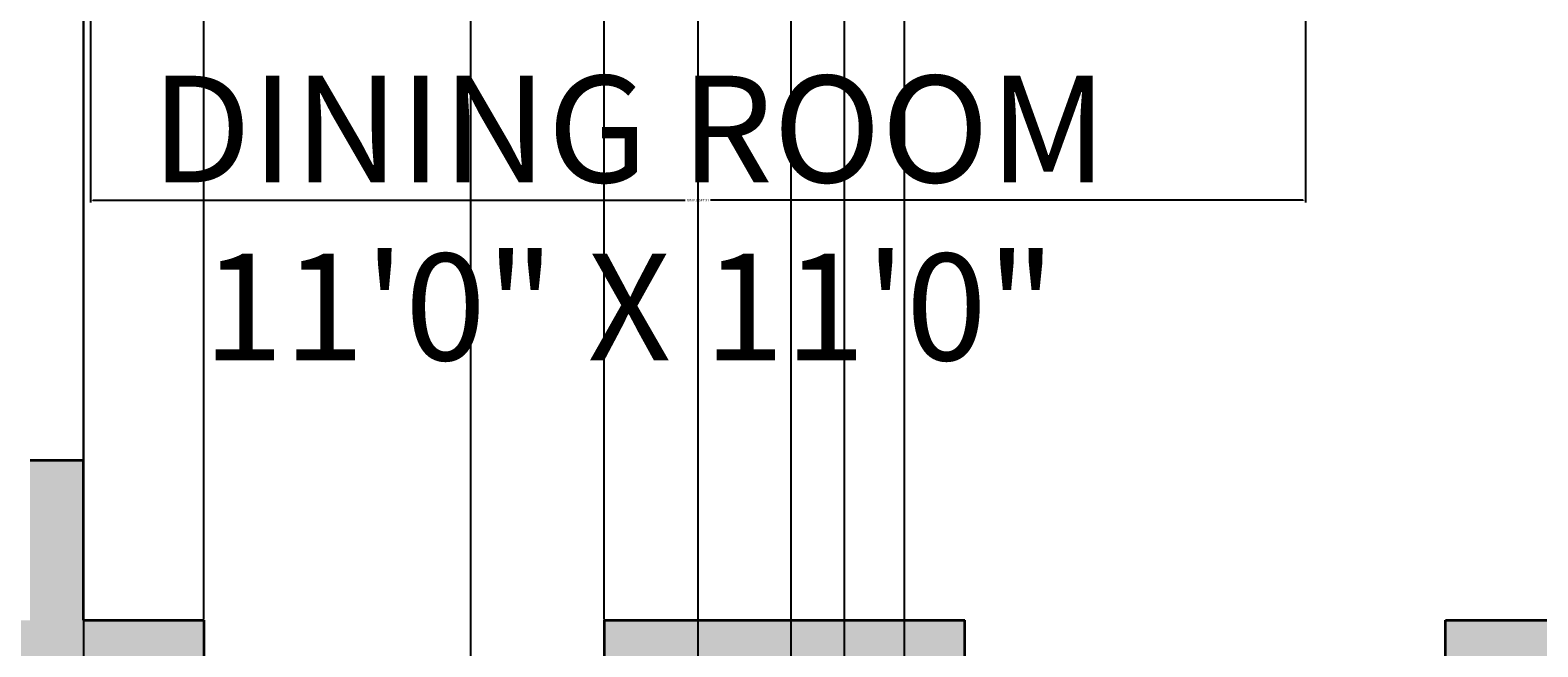
# Model space of a CAD drawing. Units: inches. Extents: x 1567 to 1964, y 1813 to 2447.
# Tile 16 of 28: x 1738 to 1851, y 2125 to 2172. Entities that reach past the tile are written whole.
import ezdxf

# ---------------------------------------------------------------- set-up
doc = ezdxf.new("R2010")
doc.units = ezdxf.units.IN
for name, color, linetype, lineweight in [('A-ANNO-DIMS', 2, 'Continuous', 18), ('A-AREA-IDEN', 7, 'Continuous', 18), ('A-WALL', 7, 'Continuous', 35)]:
    doc.layers.add(name, color=color, linetype=linetype, lineweight=lineweight)
doc.layers.add('A-WALL-PATT', color=251, linetype='Continuous', lineweight=13, true_color=0x636466)
doc.styles.get("Standard").update_dxf_attribs({"font": 'arial.ttf'})
doc.dimstyles.get("Standard").update_dxf_attribs({"dimtxt": 0.18, "dimasz": 0.18, "dimexe": 0.18, "dimexo": 0.0625, "dimgap": 0.09, "dimtad": 0, "dimtih": 1, "dimtoh": 1, "dimdec": 4, "dimzin": 0, "dimdsep": 46, "dimtxsty": 'Standard', "dimcen": 0.09, "dimadec": 0, "dimazin": 0, "dimtfac": 1, "dimtdec": 4, "dimtofl": 0, "dimtmove": 0, "dimatfit": 3, "dimfxl": 1, "dimtolj": 1, "dimtzin": 0, "dimarcsym": 0})

# ---------------------------------------------------------------- blocks, each defined once
blk = doc.blocks.new('*D27')
at = {"layer": 'A-ANNO-DIMS', "color": 0, "lineweight": -2, "transparency": 16777216}
for p, q in [((1742.95, 2172.36), (1742.95, 2158.59)), ((1833.95, 2172.36), (1833.95, 2158.59)), ((1743.13, 2158.77), (1787.5, 2158.77)), ((1833.77, 2158.77), (1789.4, 2158.77))]:
    blk.add_line(p, q, dxfattribs=at)
at = {"layer": 'A-ANNO-DIMS', "color": 0, "transparency": 16777216}
for points in [[(1743.13, 2158.8), (1743.13, 2158.74), (1742.95, 2158.77)], [(1833.77, 2158.8), (1833.77, 2158.74), (1833.95, 2158.77)]]:
    blk.add_solid(points, dxfattribs=at)
at = {"layer": 'Defpoints', "color": 0, "transparency": 16777216}
for p in [(1742.95, 2172.42), (1833.95, 2172.42), (1833.95, 2158.77)]:
    blk.add_point(p, dxfattribs=at)
at = {"layer": 'A-ANNO-DIMS', "color": 0, "transparency": 16777216, "insert": (1788.45, 2158.77), "char_height": 0.18, "attachment_point": 5}
blk.add_mtext('\\A1;DINING SET 91', dxfattribs=at)
blk = doc.blocks.new('*D47')
at = {"layer": 'A-ANNO-DIMS', "color": 0, "lineweight": -2, "transparency": 16777216}
for p, q in [((1742.43, 2331.23), (1742.43, 1813.46)), ((1788.43, 2331.23), (1788.43, 1813.46)), ((1742.61, 1813.64), (1765.21, 1813.64)), ((1788.25, 1813.64), (1765.65, 1813.64))]:
    blk.add_line(p, q, dxfattribs=at)
at = {"layer": 'A-ANNO-DIMS', "color": 0, "transparency": 16777216}
for points in [[(1742.61, 1813.67), (1742.61, 1813.61), (1742.43, 1813.64)], [(1788.25, 1813.67), (1788.25, 1813.61), (1788.43, 1813.64)]]:
    blk.add_solid(points, dxfattribs=at)
at = {"layer": 'Defpoints', "color": 0, "transparency": 16777216}
for p in [(1742.43, 2331.29), (1788.43, 2331.29), (1788.43, 1813.64)]:
    blk.add_point(p, dxfattribs=at)
at = {"layer": 'A-ANNO-DIMS', "color": 0, "transparency": 16777216, "insert": (1765.43, 1813.64), "char_height": 0.18, "attachment_point": 5}
blk.add_mtext('\\A1;46', dxfattribs=at)
blk = doc.blocks.new('*D54')
at = {"layer": 'A-ANNO-DIMS', "color": 0, "lineweight": -2, "transparency": 16777216}
for p, q in [((1711.43, 1964.35), (1711.43, 2447.12)), ((1711.61, 2446.94), (1753.21, 2446.94)), ((1795.25, 2446.94), (1753.65, 2446.94)), ((1795.43, 1964.35), (1795.43, 2447.12))]:
    blk.add_line(p, q, dxfattribs=at)
at = {"layer": 'A-ANNO-DIMS', "color": 0, "transparency": 16777216}
for points in [[(1711.61, 2446.97), (1711.61, 2446.91), (1711.43, 2446.94)], [(1795.25, 2446.97), (1795.25, 2446.91), (1795.43, 2446.94)]]:
    blk.add_solid(points, dxfattribs=at)
at = {"layer": 'Defpoints', "color": 0, "transparency": 16777216}
for p in [(1795.43, 2446.94), (1711.43, 1964.29), (1795.43, 1964.29)]:
    blk.add_point(p, dxfattribs=at)
at = {"layer": 'A-ANNO-DIMS', "color": 0, "transparency": 16777216, "insert": (1753.43, 2446.94), "char_height": 0.18, "attachment_point": 5}
blk.add_mtext('\\A1;84', dxfattribs=at)
blk = doc.blocks.new('*D55')
at = {"layer": 'A-ANNO-DIMS', "color": 0, "lineweight": -2, "transparency": 16777216}
for p, q in [((1795.43, 1964.35), (1795.43, 2447.12)), ((1795.61, 2446.94), (1797.28, 2446.94)), ((1799.25, 2446.94), (1797.58, 2446.94)), ((1799.43, 1967.35), (1799.43, 2447.12))]:
    blk.add_line(p, q, dxfattribs=at)
at = {"layer": 'A-ANNO-DIMS', "color": 0, "transparency": 16777216}
for points in [[(1795.61, 2446.97), (1795.61, 2446.91), (1795.43, 2446.94)], [(1799.25, 2446.97), (1799.25, 2446.91), (1799.43, 2446.94)]]:
    blk.add_solid(points, dxfattribs=at)
at = {"layer": 'Defpoints', "color": 0, "transparency": 16777216}
for p in [(1799.43, 2446.94), (1799.43, 1967.29), (1795.43, 1964.29)]:
    blk.add_point(p, dxfattribs=at)
at = {"layer": 'A-ANNO-DIMS', "color": 0, "transparency": 16777216, "insert": (1797.43, 2446.94), "char_height": 0.18, "attachment_point": 5}
blk.add_mtext('\\A1;4', dxfattribs=at)
blk = doc.blocks.new('*D58')
at = {"layer": 'A-ANNO-DIMS', "color": 0, "lineweight": -2, "transparency": 16777216}
for p, q in [((1742.43, 2127.35), (1742.43, 2447.12)), ((1742.61, 2446.94), (1746.78, 2446.94)), ((1751.25, 2446.94), (1747.08, 2446.94)), ((1751.43, 2127.35), (1751.43, 2447.12))]:
    blk.add_line(p, q, dxfattribs=at)
at = {"layer": 'A-ANNO-DIMS', "color": 0, "transparency": 16777216}
for points in [[(1742.61, 2446.97), (1742.61, 2446.91), (1742.43, 2446.94)], [(1751.25, 2446.97), (1751.25, 2446.91), (1751.43, 2446.94)]]:
    blk.add_solid(points, dxfattribs=at)
at = {"layer": 'Defpoints', "color": 0, "transparency": 16777216}
for p in [(1751.43, 2446.94), (1742.43, 2127.29), (1751.43, 2127.29)]:
    blk.add_point(p, dxfattribs=at)
at = {"layer": 'A-ANNO-DIMS', "color": 0, "transparency": 16777216, "insert": (1746.93, 2446.94), "char_height": 0.18, "attachment_point": 5}
blk.add_mtext('\\A1;9', dxfattribs=at)
blk = doc.blocks.new('*D59')
at = {"layer": 'A-ANNO-DIMS', "color": 0, "lineweight": -2, "transparency": 16777216}
for p, q in [((1751.43, 2127.35), (1751.43, 2447.12)), ((1751.61, 2446.94), (1766.21, 2446.94)), ((1781.25, 2446.94), (1766.65, 2446.94)), ((1781.43, 2127.35), (1781.43, 2447.12))]:
    blk.add_line(p, q, dxfattribs=at)
at = {"layer": 'A-ANNO-DIMS', "color": 0, "transparency": 16777216}
for points in [[(1751.61, 2446.97), (1751.61, 2446.91), (1751.43, 2446.94)], [(1781.25, 2446.97), (1781.25, 2446.91), (1781.43, 2446.94)]]:
    blk.add_solid(points, dxfattribs=at)
at = {"layer": 'Defpoints', "color": 0, "transparency": 16777216}
for p in [(1781.43, 2446.94), (1751.43, 2127.29), (1781.43, 2127.29)]:
    blk.add_point(p, dxfattribs=at)
at = {"layer": 'A-ANNO-DIMS', "color": 0, "transparency": 16777216, "insert": (1766.43, 2446.94), "char_height": 0.18, "attachment_point": 5}
blk.add_mtext('\\A1;30', dxfattribs=at)
blk = doc.blocks.new('*D63')
at = {"layer": 'A-ANNO-DIMS', "color": 0, "lineweight": -2, "transparency": 16777216}
for p, q in [((1735.43, 1988.35), (1735.43, 2447.12)), ((1735.61, 2446.94), (1753.21, 2446.94)), ((1771.25, 2446.94), (1753.65, 2446.94)), ((1771.43, 1988.35), (1771.43, 2447.12))]:
    blk.add_line(p, q, dxfattribs=at)
at = {"layer": 'A-ANNO-DIMS', "color": 0, "transparency": 16777216}
for points in [[(1735.61, 2446.97), (1735.61, 2446.91), (1735.43, 2446.94)], [(1771.25, 2446.97), (1771.25, 2446.91), (1771.43, 2446.94)]]:
    blk.add_solid(points, dxfattribs=at)
at = {"layer": 'Defpoints', "color": 0, "transparency": 16777216}
for p in [(1771.43, 2446.94), (1735.43, 1988.29), (1771.43, 1988.29)]:
    blk.add_point(p, dxfattribs=at)
at = {"layer": 'A-ANNO-DIMS', "color": 0, "transparency": 16777216, "insert": (1753.43, 2446.94), "char_height": 0.18, "attachment_point": 5}
blk.add_mtext('\\A1;36', dxfattribs=at)
blk = doc.blocks.new('*D70')
at = {"layer": 'A-ANNO-DIMS', "color": 0, "lineweight": -2, "transparency": 16777216}
for p, q in [((1799.43, 1967.35), (1799.43, 2447.12)), ((1799.61, 2446.94), (1801.42, 2446.94)), ((1803.75, 2446.94), (1801.94, 2446.94)), ((1803.93, 1967.35), (1803.93, 2447.12))]:
    blk.add_line(p, q, dxfattribs=at)
at = {"layer": 'A-ANNO-DIMS', "color": 0, "transparency": 16777216}
for points in [[(1799.61, 2446.97), (1799.61, 2446.91), (1799.43, 2446.94)], [(1803.75, 2446.97), (1803.75, 2446.91), (1803.93, 2446.94)]]:
    blk.add_solid(points, dxfattribs=at)
at = {"layer": 'Defpoints', "color": 0, "transparency": 16777216}
for p in [(1803.93, 2446.94), (1799.43, 1967.29), (1803.93, 1967.29)]:
    blk.add_point(p, dxfattribs=at)
at = {"layer": 'A-ANNO-DIMS', "color": 0, "transparency": 16777216, "insert": (1801.68, 2446.94), "char_height": 0.18, "attachment_point": 5}
blk.add_mtext('\\A1;4.5', dxfattribs=at)
blk = doc.blocks.new('*D71')
at = {"layer": 'A-ANNO-DIMS', "color": 0, "lineweight": -2, "transparency": 16777216}
for p, q in [((1799.43, 1910.75), (1799.43, 2447.12)), ((1799.61, 2446.94), (1861.65, 2446.94)), ((1924.25, 2446.94), (1862.21, 2446.94)), ((1924.43, 1910.75), (1924.43, 2447.12))]:
    blk.add_line(p, q, dxfattribs=at)
at = {"layer": 'A-ANNO-DIMS', "color": 0, "transparency": 16777216}
for points in [[(1799.61, 2446.97), (1799.61, 2446.91), (1799.43, 2446.94)], [(1924.25, 2446.97), (1924.25, 2446.91), (1924.43, 2446.94)]]:
    blk.add_solid(points, dxfattribs=at)
at = {"layer": 'Defpoints', "color": 0, "transparency": 16777216}
for p in [(1924.43, 2446.94), (1799.43, 1910.69), (1924.43, 1910.69)]:
    blk.add_point(p, dxfattribs=at)
at = {"layer": 'A-ANNO-DIMS', "color": 0, "transparency": 16777216, "insert": (1861.93, 2446.94), "char_height": 0.18, "attachment_point": 5}
blk.add_mtext('\\A1;125', dxfattribs=at)

msp = doc.modelspace()

# ---------------------------------------------------------------- hatches: boundary and pattern name
at = {"layer": 'A-WALL-PATT'}
h = msp.add_hatch(color=256, dxfattribs=at)
h.dxf.hatch_style = 1
h.paths.add_polyline_path([(1606.4295, 2407.29), (1654.4295, 2407.29), (1654.4295, 2416.29), (1597.4295, 2416.29), (1597.4295, 2217.29), (1606.4295, 2217.29), (1606.4295, 2259.29), (1738.4295, 2259.29), (1738.4295, 2247.29), (1742.4295, 2247.29), (1742.4295, 2259.29), (1742.4295, 2272.29), (1738.4295, 2272.29), (1738.4295, 2263.29), (1606.4295, 2263.29)])
h.paths.add_polyline_path([(1753.4295, 2416.29), (1690.4295, 2416.29), (1690.4295, 2407.29), (1738.4295, 2407.29), (1738.4295, 2308.29), (1742.4295, 2308.29), (1742.4295, 2331.29), (1746.9295, 2331.29), (1746.9295, 2335.29), (1742.4295, 2335.29), (1742.4295, 2407.29), (1753.4295, 2407.29)])
h.paths.add_polyline_path([(1840.4295, 2416.29), (1777.4295, 2416.29), (1777.4295, 2407.29), (1788.4295, 2407.29), (1788.4295, 2335.29), (1776.9295, 2335.29), (1776.9295, 2331.29), (1788.4295, 2331.29), (1788.4295, 2308.29), (1792.4295, 2308.29), (1792.4295, 2407.29), (1840.4295, 2407.29)])
h.paths.add_polyline_path([(1933.4295, 2416.29), (1876.4295, 2416.29), (1876.4295, 2407.29), (1924.4295, 2407.29), (1924.4295, 2263.29), (1792.4295, 2263.29), (1792.4295, 2272.29), (1788.4295, 2272.29), (1788.4295, 2259.29), (1872.4295, 2259.29), (1872.4295, 2171.29), (1880.9295, 2171.29), (1880.9295, 2175.29), (1876.4295, 2175.29), (1876.4295, 2259.29), (1924.4295, 2259.29), (1924.4295, 2229.29), (1933.4295, 2229.29)])
h.paths.add_polyline_path([(1933.4295, 2205.29), (1924.4295, 2205.29), (1924.4295, 2175.29), (1910.9295, 2175.29), (1910.9295, 2171.29), (1924.4295, 2171.29), (1924.4295, 2127.29), (1844.4295, 2127.29), (1844.4295, 2123.29), (1924.4295, 2123.29), (1924.4295, 2063.29), (1933.4295, 2063.29)])
h.paths.add_polyline_path([(1799.4295, 2123.29), (1808.4295, 2123.29), (1808.4295, 2127.29), (1781.4295, 2127.29), (1781.4295, 2123.29), (1795.4295, 2123.29), (1795.4295, 1964.29), (1711.4295, 1964.29), (1711.4295, 2123.29), (1751.4295, 2123.29), (1751.4295, 2127.29), (1742.4295, 2127.29), (1742.4295, 2139.29), (1738.4295, 2139.29), (1738.4295, 2127.29), (1678.4295, 2127.29), (1678.4295, 2123.29), (1702.4295, 2123.29), (1702.4295, 1913.29), (1678.4295, 1913.29), (1678.4295, 1904.29), (1711.4295, 1904.29), (1711.4295, 1960.29), (1795.4295, 1960.29), (1795.4295, 1906.69), (1929.4295, 1906.69), (1929.4295, 1848.29), (1601.4295, 1848.29), (1601.4295, 1904.29), (1630.4295, 1904.29), (1630.4295, 1913.29), (1606.4295, 1913.29), (1606.4295, 2123.29), (1630.4295, 2123.29), (1630.4295, 2127.29), (1606.4295, 2127.29), (1606.4295, 2169.29), (1597.4295, 2169.29), (1597.4295, 1844.29), (1933.4295, 1844.29), (1933.4295, 2027.29), (1924.4295, 2027.29), (1924.4295, 1967.29), (1833.9295, 1967.29), (1833.9295, 1963.29), (1924.4295, 1963.29), (1924.4295, 1910.69), (1799.4295, 1910.69), (1799.4295, 1963.29), (1803.9295, 1963.29), (1803.9295, 1967.29), (1799.4295, 1967.29)])

# ---------------------------------------------------------------- linework, layer by layer
at = {"layer": 'A-WALL'}
for p, q in [((1738.4295, 2139.29), (1742.4295, 2139.29)), ((1742.4295, 2127.29), (1742.4295, 2139.29)), ((1742.4295, 2127.29), (1751.4295, 2127.29)), ((1751.4295, 2127.29), (1751.4295, 2123.29)), ((1781.4295, 2127.29), (1781.4295, 2123.29)), ((1781.4295, 2127.29), (1808.4295, 2127.29)), ((1808.4295, 2123.29), (1808.4295, 2127.29)), ((1844.4295, 2123.29), (1844.4295, 2127.29)), ((1844.4295, 2127.29), (1924.4295, 2127.29))]:
    msp.add_line(p, q, dxfattribs=at)

# ---------------------------------------------------------------- texts
at = {"layer": 'A-AREA-IDEN', "insert": (1742.4295, 2168.1055), "char_height": 8, "attachment_point": 1}
msp.add_mtext_dynamic_manual_height_columns('\\pxqc;DINING ROOM\\P11\'0" X 11\'0"', width=81.753814, gutter_width=12.5, heights=[0], dxfattribs=at)

# ---------------------------------------------------------------- dimensions: what is measured, and where the dimension line sits
at = {"layer": 'A-ANNO-DIMS'}
for base, p1, p2, override, picture, middle in [((1795.4295, 2446.94), (1711.4295, 1964.29), (1795.4295, 1964.29), {"dimdec": 0, "dimlfac": 1, "dimrnd": 0, "dimzin": 0, "dimdsep": 46, "dimlunit": 2}, '*D54', (1753.4295, 2446.94)), ((1771.4295, 2446.94), (1735.4295, 1988.29), (1771.4295, 1988.29), {"dimdec": 0, "dimlfac": 1, "dimrnd": 0, "dimzin": 0, "dimdsep": 46, "dimlunit": 2}, '*D63', (1753.4295, 2446.94)), ((1751.4295, 2446.94), (1742.4295, 2127.29), (1751.4295, 2127.29), {"dimdec": 0, "dimlfac": 1, "dimrnd": 0, "dimzin": 0, "dimdsep": 46, "dimlunit": 2}, '*D58', (1746.9295, 2446.94)), ((1781.4295, 2446.94), (1751.4295, 2127.29), (1781.4295, 2127.29), {"dimdec": 0, "dimlfac": 1, "dimrnd": 0, "dimzin": 0, "dimdsep": 46, "dimlunit": 2}, '*D59', (1766.4295, 2446.94)), ((1799.4295, 2446.94), (1795.4295, 1964.29), (1799.4295, 1967.29), {"dimdec": 0, "dimlfac": 1, "dimrnd": 0, "dimzin": 0, "dimdsep": 46, "dimlunit": 2}, '*D55', (1797.4295, 2446.94)), ((1803.9295, 2446.94), (1799.4295, 1967.29), (1803.9295, 1967.29), {"dimdec": 1, "dimlfac": 1, "dimrnd": 0, "dimzin": 0, "dimdsep": 46, "dimlunit": 2}, '*D70', (1801.6795, 2446.94)), ((1924.4295, 2446.94), (1799.4295, 1910.69), (1924.4295, 1910.69), {"dimdec": 0, "dimlfac": 1, "dimrnd": 0, "dimzin": 0, "dimdsep": 46, "dimlunit": 2}, '*D71', (1861.9295, 2446.94)), ((1788.4295, 1813.64), (1742.4295, 2331.29), (1788.4295, 2331.29), {"dimdec": 0, "dimlfac": 1, "dimrnd": 0, "dimzin": 0, "dimdsep": 46, "dimlunit": 2}, '*D47', (1765.4295, 1813.64))]:
    dim = msp.add_linear_dim(base=base, p1=p1, p2=p2, dimstyle='Standard', override=override, dxfattribs=at)
    dim.commit()
    dim.dimension.update_dxf_attribs({"geometry": picture, "text_midpoint": middle})
dim = msp.add_linear_dim(base=(1833.9511, 2158.7697), p1=(1742.9511, 2172.4197), p2=(1833.9511, 2172.4197), text='DINING SET <>', dimstyle='Standard', override={"dimdec": 0, "dimlfac": 1, "dimrnd": 0, "dimzin": 0, "dimdsep": 46, "dimlunit": 2}, dxfattribs=at)
dim.commit()
dim.dimension.update_dxf_attribs({"geometry": '*D27', "text_midpoint": (1788.4511, 2158.7697)})

doc.saveas('drawing.dxf')
